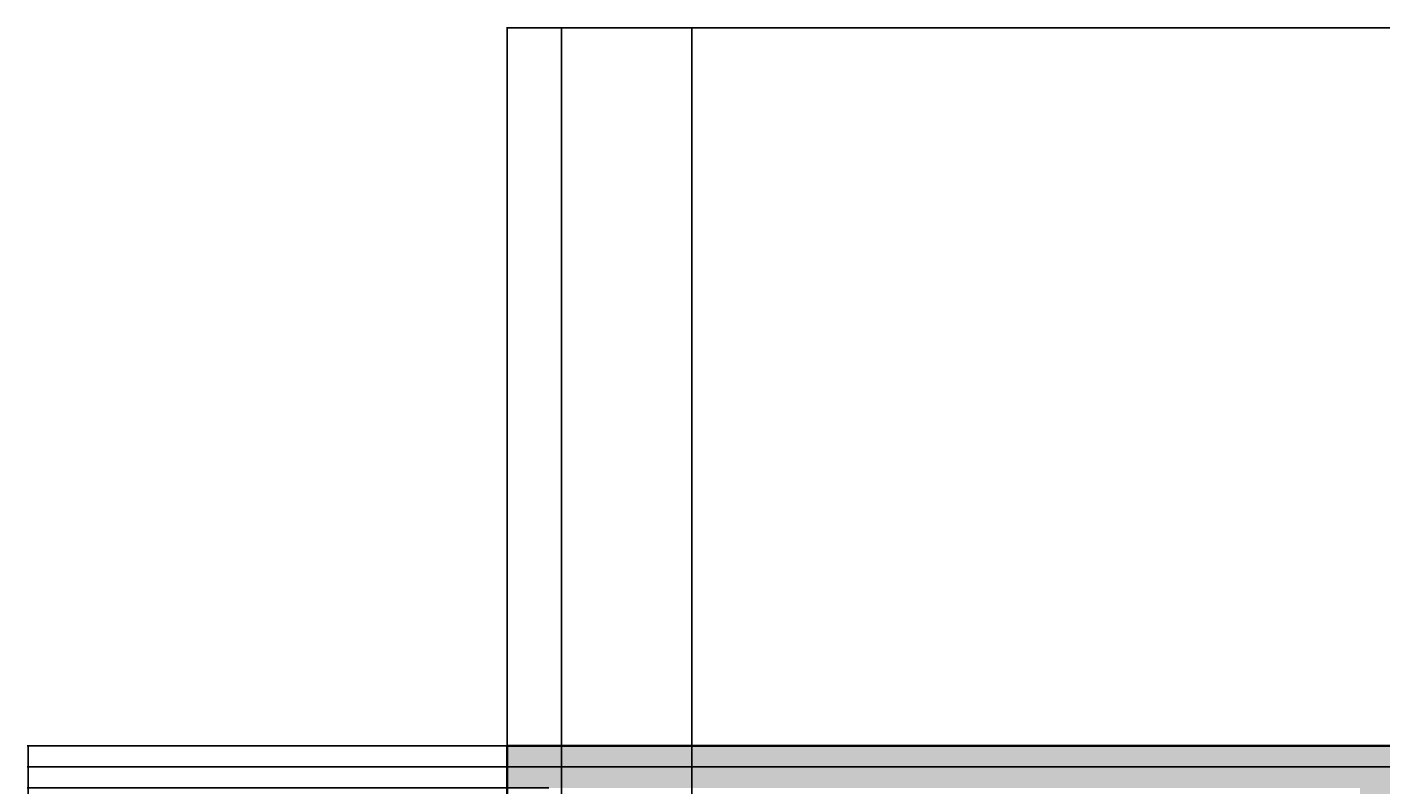
# Model space of a CAD drawing. Units: inches. Extents: x 5716 to 6907, y 12769 to 13594.
# Tile 7 of 17: x 5716 to 6007, y 13432 to 13594. Entities that reach past the tile are written whole.
import ezdxf

# ---------------------------------------------------------------- set-up
doc = ezdxf.new("R2010")
doc.units = ezdxf.units.IN
for name, color, linetype, lineweight in [('A-ANNO-DIMS', 2, 'Continuous', 18), ('A-WALL', 7, 'Continuous', 35), ('A-WALL-PATT', 252, 'Continuous', 13)]:
    doc.layers.add(name, color=color, linetype=linetype, lineweight=lineweight)
doc.styles.get("Standard").update_dxf_attribs({"font": 'arial.ttf'})
doc.dimstyles.get("Standard").update_dxf_attribs({"dimtxt": 0.18, "dimasz": 0.18, "dimexe": 0.18, "dimexo": 0.0625, "dimgap": 0.09, "dimtad": 0, "dimtih": 1, "dimtoh": 1, "dimdec": 4, "dimzin": 0, "dimdsep": 46, "dimtxsty": 'Standard', "dimcen": 0.09, "dimadec": 0, "dimazin": 0, "dimtfac": 1, "dimtdec": 4, "dimtofl": 0, "dimtmove": 0, "dimatfit": 3, "dimfxl": 1, "dimtolj": 1, "dimtzin": 0, "dimarcsym": 0})

# ---------------------------------------------------------------- blocks, each defined once
blk = doc.blocks.new('*D50')
at = {"layer": 'A-ANNO-DIMS', "color": 0, "lineweight": -2, "transparency": 16777216}
for p, q in [((5818.96, 13440.15), (5716.04, 13440.15)), ((5716.22, 13439.97), (5716.22, 13140.83)), ((5716.22, 12841.33), (5716.22, 13140.47)), ((5818.96, 12841.15), (5716.04, 12841.15))]:
    blk.add_line(p, q, dxfattribs=at)
at = {"layer": 'A-ANNO-DIMS', "color": 0, "transparency": 16777216}
for points in [[(5716.19, 13439.97), (5716.25, 13439.97), (5716.22, 13440.15)], [(5716.19, 12841.33), (5716.25, 12841.33), (5716.22, 12841.15)]]:
    blk.add_solid(points, dxfattribs=at)
at = {"layer": 'Defpoints', "color": 0, "transparency": 16777216}
for p in [(5716.22, 13440.15), (5819.02, 13440.15), (5819.02, 12841.15)]:
    blk.add_point(p, dxfattribs=at)
at = {"layer": 'A-ANNO-DIMS', "color": 0, "transparency": 16777216, "insert": (5716.22, 13140.65), "char_height": 0.18, "attachment_point": 5}
blk.add_mtext('\\A1;599', dxfattribs=at)
blk = doc.blocks.new('*D51')
at = {"layer": 'A-ANNO-DIMS', "color": 0, "lineweight": -2, "transparency": 16777216}
for p, q in [((5819.02, 13440.21), (5819.02, 13594.38)), ((5819.2, 13594.2), (6033.23, 13594.2)), ((6247.84, 13594.2), (6033.82, 13594.2)), ((6248.02, 13194.21), (6248.02, 13594.38))]:
    blk.add_line(p, q, dxfattribs=at)
at = {"layer": 'A-ANNO-DIMS', "color": 0, "transparency": 16777216}
for points in [[(5819.2, 13594.23), (5819.2, 13594.17), (5819.02, 13594.2)], [(6247.84, 13594.23), (6247.84, 13594.17), (6248.02, 13594.2)]]:
    blk.add_solid(points, dxfattribs=at)
at = {"layer": 'Defpoints', "color": 0, "transparency": 16777216}
for p in [(6248.02, 13594.2), (5819.02, 13440.15), (6248.02, 13194.15)]:
    blk.add_point(p, dxfattribs=at)
at = {"layer": 'A-ANNO-DIMS', "color": 0, "transparency": 16777216, "insert": (6033.52, 13594.2), "char_height": 0.18, "attachment_point": 5}
blk.add_mtext('\\A1;429', dxfattribs=at)
blk = doc.blocks.new('*D52')
at = {"layer": 'A-ANNO-DIMS', "color": 0, "lineweight": -2, "transparency": 16777216}
for p, q in [((6267.34, 13440.15), (5716.04, 13440.15)), ((5716.22, 13439.97), (5716.22, 13140.83)), ((5716.22, 12841.33), (5716.22, 13140.47)), ((6267.34, 12841.15), (5716.04, 12841.15))]:
    blk.add_line(p, q, dxfattribs=at)
at = {"layer": 'A-ANNO-DIMS', "color": 0, "transparency": 16777216}
for points in [[(5716.19, 13439.97), (5716.25, 13439.97), (5716.22, 13440.15)], [(5716.19, 12841.33), (5716.25, 12841.33), (5716.22, 12841.15)]]:
    blk.add_solid(points, dxfattribs=at)
at = {"layer": 'Defpoints', "color": 0, "transparency": 16777216}
for p in [(6267.41, 13440.15), (5716.22, 12841.15), (6267.41, 12841.15)]:
    blk.add_point(p, dxfattribs=at)
at = {"layer": 'A-ANNO-DIMS', "color": 0, "transparency": 16777216, "insert": (5716.22, 13140.65), "char_height": 0.18, "attachment_point": 5}
blk.add_mtext('\\A1;599', dxfattribs=at)
blk = doc.blocks.new('*D58')
at = {"layer": 'A-ANNO-DIMS', "color": 0, "lineweight": -2, "transparency": 16777216}
for p, q in [((6736.67, 13435.65), (5716.04, 13435.65)), ((5716.22, 13435.47), (5716.22, 13365.33)), ((5716.22, 13294.83), (5716.22, 13364.97)), ((6736.67, 13294.65), (5716.04, 13294.65))]:
    blk.add_line(p, q, dxfattribs=at)
at = {"layer": 'A-ANNO-DIMS', "color": 0, "transparency": 16777216}
for points in [[(5716.19, 13435.47), (5716.25, 13435.47), (5716.22, 13435.65)], [(5716.19, 13294.83), (5716.25, 13294.83), (5716.22, 13294.65)]]:
    blk.add_solid(points, dxfattribs=at)
at = {"layer": 'Defpoints', "color": 0, "transparency": 16777216}
for p in [(6736.73, 13435.65), (5716.22, 13294.65), (6736.73, 13294.65)]:
    blk.add_point(p, dxfattribs=at)
at = {"layer": 'A-ANNO-DIMS', "color": 0, "transparency": 16777216, "insert": (5716.22, 13365.15), "char_height": 0.18, "attachment_point": 5}
blk.add_mtext('\\A1;141', dxfattribs=at)
blk = doc.blocks.new('*D65')
at = {"layer": 'A-ANNO-DIMS', "color": 0, "lineweight": -2, "transparency": 16777216}
for p, q in [((5818.96, 13440.15), (5716.04, 13440.15)), ((5716.22, 13439.97), (5716.22, 13435.83)), ((5716.22, 13431.33), (5716.22, 13435.47)), ((5827.96, 13431.15), (5716.04, 13431.15))]:
    blk.add_line(p, q, dxfattribs=at)
at = {"layer": 'A-ANNO-DIMS', "color": 0, "transparency": 16777216}
for points in [[(5716.19, 13439.97), (5716.25, 13439.97), (5716.22, 13440.15)], [(5716.19, 13431.33), (5716.25, 13431.33), (5716.22, 13431.15)]]:
    blk.add_solid(points, dxfattribs=at)
at = {"layer": 'Defpoints', "color": 0, "transparency": 16777216}
for p in [(5819.02, 13440.15), (5716.22, 13431.15), (5828.02, 13431.15)]:
    blk.add_point(p, dxfattribs=at)
at = {"layer": 'A-ANNO-DIMS', "color": 0, "transparency": 16777216, "insert": (5716.22, 13435.65), "char_height": 0.18, "attachment_point": 5}
blk.add_mtext('\\A1;9', dxfattribs=at)
blk = doc.blocks.new('*D75')
at = {"layer": 'A-ANNO-DIMS', "color": 0, "lineweight": -2, "transparency": 16777216}
for p, q in [((5830.67, 13257.62), (5830.67, 13594.38)), ((5830.85, 13594.2), (5844.45, 13594.2)), ((5858.49, 13594.2), (5844.89, 13594.2)), ((5858.67, 13247.12), (5858.67, 13594.38))]:
    blk.add_line(p, q, dxfattribs=at)
at = {"layer": 'A-ANNO-DIMS', "color": 0, "transparency": 16777216}
for points in [[(5830.85, 13594.23), (5830.85, 13594.17), (5830.67, 13594.2)], [(5858.49, 13594.23), (5858.49, 13594.17), (5858.67, 13594.2)]]:
    blk.add_solid(points, dxfattribs=at)
at = {"layer": 'Defpoints', "color": 0, "transparency": 16777216}
for p in [(5858.67, 13594.2), (5830.67, 13257.56), (5858.67, 13247.06)]:
    blk.add_point(p, dxfattribs=at)
at = {"layer": 'A-ANNO-DIMS', "color": 0, "transparency": 16777216, "insert": (5844.67, 13594.2), "char_height": 0.18, "attachment_point": 5}
blk.add_mtext('\\A1;28', dxfattribs=at)

msp = doc.modelspace()

# ---------------------------------------------------------------- hatches: boundary and pattern name
at = {"layer": 'A-WALL-PATT'}
h = msp.add_hatch(color=256, dxfattribs=at)
h.dxf.hatch_style = 1
h.paths.add_polyline_path([(6188.02, 13440.15), (5819.02, 13440.15), (5819.02, 13431.15), (6002.02, 13431.15), (6002.02, 13290.15), (6011.02, 13290.15), (6011.02, 13431.15), (6188.02, 13431.15)])

# ---------------------------------------------------------------- linework, layer by layer
at = {"layer": 'A-WALL'}
for q in [(6188.02, 13440.15), (5819.02, 12841.15)]:
    msp.add_line((5819.02, 13440.15), q, dxfattribs=at)

# ---------------------------------------------------------------- dimensions: what is measured, and where the dimension line sits
at = {"layer": 'A-ANNO-DIMS'}
for base, p1, p2, picture, middle in [((6248.02, 13594.2), (5819.02, 13440.15), (6248.02, 13194.15), '*D51', (6033.52, 13594.2)), ((5858.67, 13594.2), (5830.67, 13257.56), (5858.67, 13247.06), '*D75', (5844.67, 13594.2))]:
    dim = msp.add_linear_dim(base=base, p1=p1, p2=p2, dimstyle='Standard', override={"dimdec": 0, "dimlfac": 1, "dimrnd": 0, "dimzin": 0, "dimdsep": 46, "dimlunit": 2}, dxfattribs=at)
    dim.commit()
    dim.dimension.update_dxf_attribs({"geometry": picture, "text_midpoint": middle})
for base, p1, p2, picture, middle in [((5716.22, 13440.15), (5819.02, 12841.15), (5819.02, 13440.15), '*D50', (5716.22, 13140.65)), ((5716.22, 12841.15), (6267.41, 13440.15), (6267.41, 12841.15), '*D52', (5716.22, 13140.65)), ((5716.22, 13431.15), (5819.02, 13440.15), (5828.02, 13431.15), '*D65', (5716.22, 13435.65)), ((5716.22, 13294.65), (6736.73, 13435.65), (6736.73, 13294.65), '*D58', (5716.22, 13365.15))]:
    dim = msp.add_linear_dim(base=base, p1=p1, p2=p2, angle=90, dimstyle='Standard', override={"dimdec": 0, "dimlfac": 1, "dimrnd": 0, "dimzin": 0, "dimdsep": 46, "dimlunit": 2}, dxfattribs=at)
    dim.commit()
    dim.dimension.update_dxf_attribs({"geometry": picture, "text_midpoint": middle})

doc.saveas('drawing.dxf')
